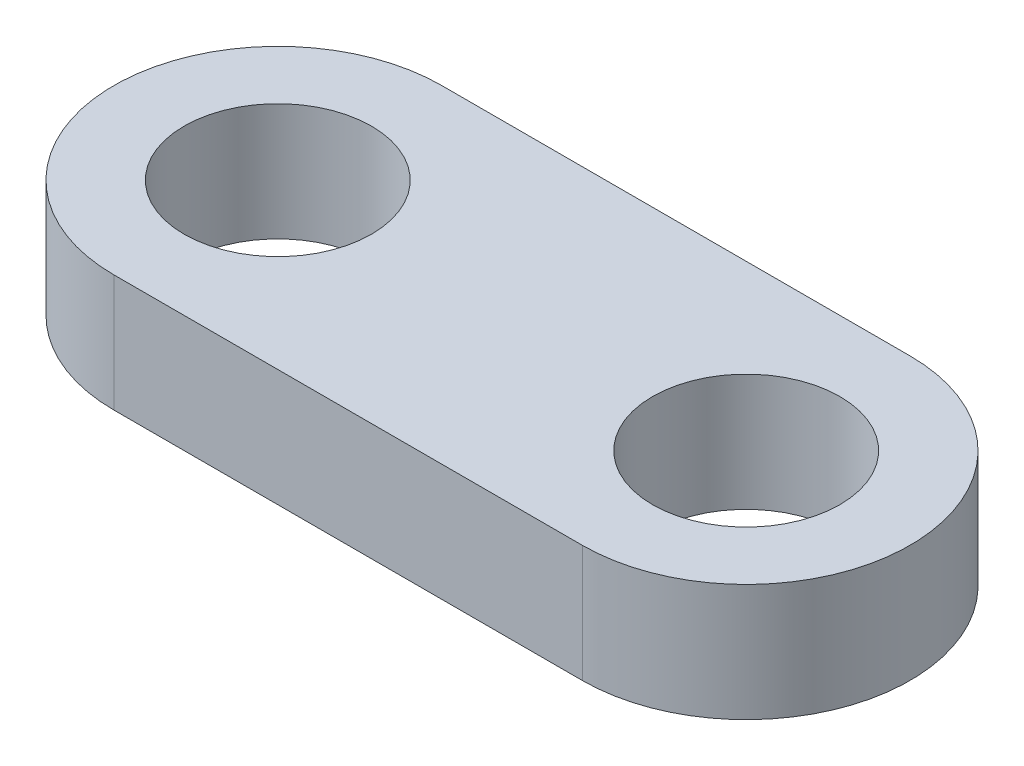
ISO-10303-21;
HEADER;
FILE_DESCRIPTION(('STEP AP214'),'2;1');
FILE_NAME('part.step','',(''),(''),'','','');
FILE_SCHEMA(('AUTOMOTIVE_DESIGN { 1 0 10303 214 1 1 1 1 }'));
ENDSEC;
DATA;
#1=APPLICATION_CONTEXT('core data for automotive mechanical design processes');
#2=APPLICATION_PROTOCOL_DEFINITION('international standard','automotive_design',2000,#1);
#3=PRODUCT_CONTEXT('',#1,'mechanical');
#4=PRODUCT('Part','Part','',(#3));
#5=PRODUCT_RELATED_PRODUCT_CATEGORY('part','',(#4));
#6=PRODUCT_DEFINITION_FORMATION('','',#4);
#7=PRODUCT_DEFINITION_CONTEXT('part definition',#1,'design');
#8=PRODUCT_DEFINITION('design','',#6,#7);
#9=PRODUCT_DEFINITION_SHAPE('','',#8);
#10=(LENGTH_UNIT() NAMED_UNIT(*) SI_UNIT(.MILLI.,.METRE.));
#11=(NAMED_UNIT(*) PLANE_ANGLE_UNIT() SI_UNIT($,.RADIAN.));
#12=(NAMED_UNIT(*) SI_UNIT($,.STERADIAN.) SOLID_ANGLE_UNIT());
#13=UNCERTAINTY_MEASURE_WITH_UNIT(LENGTH_MEASURE(1.E-05),#10,'distance_accuracy_value','');
#14=(GEOMETRIC_REPRESENTATION_CONTEXT(3) GLOBAL_UNCERTAINTY_ASSIGNED_CONTEXT((#13)) GLOBAL_UNIT_ASSIGNED_CONTEXT((#10,
#11,#12)) REPRESENTATION_CONTEXT('',''));
#15=CARTESIAN_POINT('',(0.,0.,0.));
#16=DIRECTION('',(0.,0.,1.));
#17=DIRECTION('',(1.,0.,0.));
#18=AXIS2_PLACEMENT_3D('',#15,#16,#17);
#19=CARTESIAN_POINT('',(-10.,2.5,0.));
#20=DIRECTION('',(0.,-1.,0.));
#21=DIRECTION('',(0.,0.,-1.));
#22=AXIS2_PLACEMENT_3D('',#19,#20,#21);
#23=CYLINDRICAL_SURFACE('',#22,7.);
#24=CARTESIAN_POINT('',(-10.,-2.5,0.));
#25=DIRECTION('',(0.,1.,0.));
#26=DIRECTION('',(0.,0.,1.));
#27=AXIS2_PLACEMENT_3D('',#24,#25,#26);
#28=CIRCLE('',#27,7.);
#29=CARTESIAN_POINT('',(-10.,-2.5,-7.));
#30=VERTEX_POINT('',#29);
#31=CARTESIAN_POINT('',(-10.,-2.5,7.));
#32=VERTEX_POINT('',#31);
#33=EDGE_CURVE('E102',#30,#32,#28,.T.);
#34=ORIENTED_EDGE('',*,*,#33,.T.);
#35=DIRECTION('',(0.,-1.,0.));
#36=VECTOR('',#35,1.);
#37=CARTESIAN_POINT('',(-10.,2.5,7.));
#38=LINE('',#37,#36);
#39=CARTESIAN_POINT('',(-10.,2.5,7.));
#40=VERTEX_POINT('',#39);
#41=EDGE_CURVE('E11',#40,#32,#38,.T.);
#42=ORIENTED_EDGE('',*,*,#41,.F.);
#43=CARTESIAN_POINT('',(-10.,2.5,0.));
#44=DIRECTION('',(0.,1.,0.));
#45=DIRECTION('',(0.,0.,1.));
#46=AXIS2_PLACEMENT_3D('',#43,#44,#45);
#47=CIRCLE('',#46,7.);
#48=CARTESIAN_POINT('',(-10.,2.5,-7.));
#49=VERTEX_POINT('',#48);
#50=EDGE_CURVE('E95',#49,#40,#47,.T.);
#51=ORIENTED_EDGE('',*,*,#50,.F.);
#52=DIRECTION('',(0.,-1.,0.));
#53=VECTOR('',#52,1.);
#54=CARTESIAN_POINT('',(-10.,2.5,-7.));
#55=LINE('',#54,#53);
#56=EDGE_CURVE('E99',#49,#30,#55,.T.);
#57=ORIENTED_EDGE('',*,*,#56,.T.);
#58=EDGE_LOOP('',(#34,#42,#51,#57));
#59=FACE_BOUND('',#58,.T.);
#60=ADVANCED_FACE('F41',(#59),#23,.T.);
#61=CARTESIAN_POINT('',(-10.,2.5,7.));
#62=DIRECTION('',(0.,0.,-1.));
#63=DIRECTION('',(-1.,0.,0.));
#64=AXIS2_PLACEMENT_3D('',#61,#62,#63);
#65=PLANE('',#64);
#66=DIRECTION('',(1.,0.,0.));
#67=VECTOR('',#66,1.);
#68=CARTESIAN_POINT('',(-10.,-2.5,7.));
#69=LINE('',#68,#67);
#70=CARTESIAN_POINT('',(10.,-2.5,7.));
#71=VERTEX_POINT('',#70);
#72=EDGE_CURVE('E96',#32,#71,#69,.T.);
#73=ORIENTED_EDGE('',*,*,#72,.T.);
#74=DIRECTION('',(0.,-1.,0.));
#75=VECTOR('',#74,1.);
#76=CARTESIAN_POINT('',(10.,2.5,7.));
#77=LINE('',#76,#75);
#78=CARTESIAN_POINT('',(10.,2.5,7.));
#79=VERTEX_POINT('',#78);
#80=EDGE_CURVE('E47',#79,#71,#77,.T.);
#81=ORIENTED_EDGE('',*,*,#80,.F.);
#82=DIRECTION('',(1.,0.,0.));
#83=VECTOR('',#82,1.);
#84=CARTESIAN_POINT('',(-10.,2.5,7.));
#85=LINE('',#84,#83);
#86=EDGE_CURVE('E87',#40,#79,#85,.T.);
#87=ORIENTED_EDGE('',*,*,#86,.F.);
#88=ORIENTED_EDGE('',*,*,#41,.T.);
#89=EDGE_LOOP('',(#73,#81,#87,#88));
#90=FACE_BOUND('',#89,.T.);
#91=ADVANCED_FACE('F92',(#90),#65,.F.);
#92=CARTESIAN_POINT('',(10.,2.5,0.));
#93=DIRECTION('',(0.,-1.,0.));
#94=DIRECTION('',(0.,0.,-1.));
#95=AXIS2_PLACEMENT_3D('',#92,#93,#94);
#96=CYLINDRICAL_SURFACE('',#95,7.);
#97=CARTESIAN_POINT('',(10.,-2.5,0.));
#98=DIRECTION('',(0.,1.,0.));
#99=DIRECTION('',(0.,0.,1.));
#100=AXIS2_PLACEMENT_3D('',#97,#98,#99);
#101=CIRCLE('',#100,7.);
#102=CARTESIAN_POINT('',(10.,-2.5,-7.));
#103=VERTEX_POINT('',#102);
#104=EDGE_CURVE('E74',#71,#103,#101,.T.);
#105=ORIENTED_EDGE('',*,*,#104,.T.);
#106=DIRECTION('',(0.,-1.,0.));
#107=VECTOR('',#106,1.);
#108=CARTESIAN_POINT('',(10.,2.5,-7.));
#109=LINE('',#108,#107);
#110=CARTESIAN_POINT('',(10.,2.5,-7.));
#111=VERTEX_POINT('',#110);
#112=EDGE_CURVE('E100',#111,#103,#109,.T.);
#113=ORIENTED_EDGE('',*,*,#112,.F.);
#114=CARTESIAN_POINT('',(10.,2.5,0.));
#115=DIRECTION('',(0.,1.,0.));
#116=DIRECTION('',(0.,0.,1.));
#117=AXIS2_PLACEMENT_3D('',#114,#115,#116);
#118=CIRCLE('',#117,7.);
#119=EDGE_CURVE('E89',#79,#111,#118,.T.);
#120=ORIENTED_EDGE('',*,*,#119,.F.);
#121=ORIENTED_EDGE('',*,*,#80,.T.);
#122=EDGE_LOOP('',(#105,#113,#120,#121));
#123=FACE_BOUND('',#122,.T.);
#124=ADVANCED_FACE('F98',(#123),#96,.T.);
#125=CARTESIAN_POINT('',(-10.,2.5,-7.));
#126=DIRECTION('',(0.,0.,1.));
#127=DIRECTION('',(1.,0.,0.));
#128=AXIS2_PLACEMENT_3D('',#125,#126,#127);
#129=PLANE('',#128);
#130=DIRECTION('',(-1.,0.,0.));
#131=VECTOR('',#130,1.);
#132=CARTESIAN_POINT('',(-10.,-2.5,-7.));
#133=LINE('',#132,#131);
#134=EDGE_CURVE('E77',#103,#30,#133,.T.);
#135=ORIENTED_EDGE('',*,*,#134,.T.);
#136=ORIENTED_EDGE('',*,*,#56,.F.);
#137=DIRECTION('',(-1.,0.,0.));
#138=VECTOR('',#137,1.);
#139=CARTESIAN_POINT('',(-10.,2.5,-7.));
#140=LINE('',#139,#138);
#141=EDGE_CURVE('E60',#111,#49,#140,.T.);
#142=ORIENTED_EDGE('',*,*,#141,.F.);
#143=ORIENTED_EDGE('',*,*,#112,.T.);
#144=EDGE_LOOP('',(#135,#136,#142,#143));
#145=FACE_BOUND('',#144,.T.);
#146=ADVANCED_FACE('F115',(#145),#129,.F.);
#147=CARTESIAN_POINT('',(-10.,2.5,0.));
#148=DIRECTION('',(0.,1.,0.));
#149=DIRECTION('',(0.,0.,1.));
#150=AXIS2_PLACEMENT_3D('',#147,#148,#149);
#151=PLANE('',#150);
#152=CARTESIAN_POINT('',(-10.,2.5,0.));
#153=DIRECTION('',(0.,1.,0.));
#154=DIRECTION('',(0.,0.,1.));
#155=AXIS2_PLACEMENT_3D('',#152,#153,#154);
#156=CIRCLE('',#155,4.);
#157=CARTESIAN_POINT('',(-10.,2.5,4.));
#158=VERTEX_POINT('',#157);
#159=EDGE_CURVE('E123',#158,#158,#156,.T.);
#160=ORIENTED_EDGE('',*,*,#159,.F.);
#161=EDGE_LOOP('',(#160));
#162=FACE_BOUND('',#161,.T.);
#163=CARTESIAN_POINT('',(10.,2.5,0.));
#164=DIRECTION('',(0.,1.,0.));
#165=DIRECTION('',(0.,0.,1.));
#166=AXIS2_PLACEMENT_3D('',#163,#164,#165);
#167=CIRCLE('',#166,4.);
#168=CARTESIAN_POINT('',(10.,2.5,4.));
#169=VERTEX_POINT('',#168);
#170=EDGE_CURVE('E124',#169,#169,#167,.T.);
#171=ORIENTED_EDGE('',*,*,#170,.F.);
#172=EDGE_LOOP('',(#171));
#173=FACE_BOUND('',#172,.T.);
#174=ORIENTED_EDGE('',*,*,#50,.T.);
#175=ORIENTED_EDGE('',*,*,#86,.T.);
#176=ORIENTED_EDGE('',*,*,#119,.T.);
#177=ORIENTED_EDGE('',*,*,#141,.T.);
#178=EDGE_LOOP('',(#174,#175,#176,#177));
#179=FACE_BOUND('',#178,.T.);
#180=ADVANCED_FACE('F86',(#162,#173,#179),#151,.T.);
#181=CARTESIAN_POINT('',(-10.,-2.5,0.));
#182=DIRECTION('',(0.,1.,0.));
#183=DIRECTION('',(0.,0.,1.));
#184=AXIS2_PLACEMENT_3D('',#181,#182,#183);
#185=PLANE('',#184);
#186=CARTESIAN_POINT('',(-10.,-2.5,0.));
#187=DIRECTION('',(0.,1.,0.));
#188=DIRECTION('',(0.,0.,1.));
#189=AXIS2_PLACEMENT_3D('',#186,#187,#188);
#190=CIRCLE('',#189,4.);
#191=CARTESIAN_POINT('',(-10.,-2.5,4.));
#192=VERTEX_POINT('',#191);
#193=EDGE_CURVE('E110',#192,#192,#190,.T.);
#194=ORIENTED_EDGE('',*,*,#193,.T.);
#195=EDGE_LOOP('',(#194));
#196=FACE_BOUND('',#195,.T.);
#197=CARTESIAN_POINT('',(10.,-2.5,0.));
#198=DIRECTION('',(0.,1.,0.));
#199=DIRECTION('',(0.,0.,1.));
#200=AXIS2_PLACEMENT_3D('',#197,#198,#199);
#201=CIRCLE('',#200,4.);
#202=CARTESIAN_POINT('',(10.,-2.5,4.));
#203=VERTEX_POINT('',#202);
#204=EDGE_CURVE('E120',#203,#203,#201,.T.);
#205=ORIENTED_EDGE('',*,*,#204,.T.);
#206=EDGE_LOOP('',(#205));
#207=FACE_BOUND('',#206,.T.);
#208=ORIENTED_EDGE('',*,*,#33,.F.);
#209=ORIENTED_EDGE('',*,*,#134,.F.);
#210=ORIENTED_EDGE('',*,*,#104,.F.);
#211=ORIENTED_EDGE('',*,*,#72,.F.);
#212=EDGE_LOOP('',(#208,#209,#210,#211));
#213=FACE_BOUND('',#212,.T.);
#214=ADVANCED_FACE('F113',(#196,#207,#213),#185,.F.);
#215=CARTESIAN_POINT('',(10.,-2.5,0.));
#216=DIRECTION('',(0.,1.,0.));
#217=DIRECTION('',(0.,0.,1.));
#218=AXIS2_PLACEMENT_3D('',#215,#216,#217);
#219=CYLINDRICAL_SURFACE('',#218,4.);
#220=ORIENTED_EDGE('',*,*,#204,.F.);
#221=EDGE_LOOP('',(#220));
#222=FACE_BOUND('',#221,.T.);
#223=ORIENTED_EDGE('',*,*,#170,.T.);
#224=EDGE_LOOP('',(#223));
#225=FACE_BOUND('',#224,.T.);
#226=ADVANCED_FACE('F132',(#222,#225),#219,.F.);
#227=CARTESIAN_POINT('',(-10.,-2.5,0.));
#228=DIRECTION('',(0.,1.,0.));
#229=DIRECTION('',(0.,0.,1.));
#230=AXIS2_PLACEMENT_3D('',#227,#228,#229);
#231=CYLINDRICAL_SURFACE('',#230,4.);
#232=ORIENTED_EDGE('',*,*,#193,.F.);
#233=EDGE_LOOP('',(#232));
#234=FACE_BOUND('',#233,.T.);
#235=ORIENTED_EDGE('',*,*,#159,.T.);
#236=EDGE_LOOP('',(#235));
#237=FACE_BOUND('',#236,.T.);
#238=ADVANCED_FACE('F131',(#234,#237),#231,.F.);
#239=CLOSED_SHELL('',(#60,#91,#124,#146,#180,#214,#226,#238));
#240=MANIFOLD_SOLID_BREP('B2',#239);
#241=ADVANCED_BREP_SHAPE_REPRESENTATION('',(#18,#240),#14);
#242=SHAPE_DEFINITION_REPRESENTATION(#9,#241);
ENDSEC;
END-ISO-10303-21;
